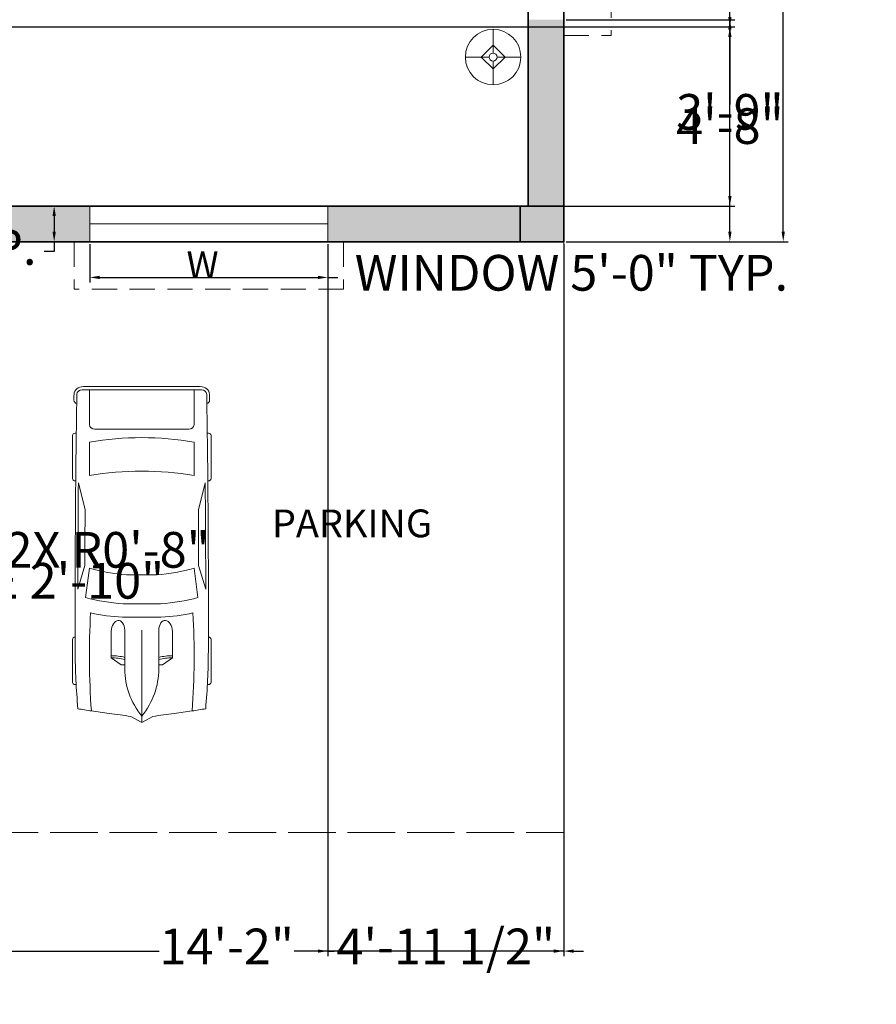
# Model space of a CAD drawing. Units: inches. Extents: x 9689 to 10369, y 10965 to 11626.
# Tile 9 of 11: x 10107 to 10323, y 10965 to 11214. Entities that reach past the tile are written whole.
import ezdxf

# ---------------------------------------------------------------- set-up
doc = ezdxf.new("R2010")
doc.units = ezdxf.units.IN
doc.linetypes.add('ACAD_ISO02W100', pattern=[15, 12, -3])
doc.linetypes.add('DASHED2', pattern=[9.525, 6.35, -3.175])
for name, color, linetype, lineweight in [('A-ANNO-DIMS', 2, 'Continuous', 18), ('A-ANNO-TEXT', 7, 'Continuous', 18), ('A-AREA-IDEN', 7, 'Continuous', 18), ('A-COLS', 7, 'Continuous', 35), ('A-FURN', 8, 'Continuous', 18), ('A-GLAZ', 4, 'Continuous', 18), ('A-GLAZ-OVHD', 4, 'DASHED2', 13), ('A-WALL', 7, 'Continuous', 35), ('A-WALL-PATT', 252, 'Continuous', 13), ('C-PARK', 7, 'ACAD_ISO02W100', 18), ('C-PARK-VEHI', 8, 'Continuous', 13)]:
    doc.layers.add(name, color=color, linetype=linetype, lineweight=lineweight)
doc.layers.add('A-COLS-PATT', color=18, linetype='Continuous', lineweight=13, true_color=0x000000)
doc.styles.get("Standard").update_dxf_attribs({"font": 'arial.ttf'})
doc.dimstyles.new('ISO-25', dxfattribs={"dimtxt": 9, "dimasz": 2.5, "dimexe": 1.25, "dimexo": 0.625, "dimgap": 2, "dimtad": 0, "dimtih": 1, "dimtoh": 1, "dimdec": 1, "dimlunit": 4, "dimtxsty": 'Standard', "dimcen": 2.5, "dimadec": 0, "dimazin": 0, "dimtfac": 0.5, "dimtdec": 1, "dimtmove": 0, "dimatfit": 3, "dimfxl": 1, "dimarcsym": 0})

# ---------------------------------------------------------------- blocks, each defined once
blk = doc.blocks.new('Lamp - Table')
for p, q in [((0, 7), (0, 1)), ((0, 3), (-3, 0)), ((3, 0), (0, 3)), ((-1, 0), (-7, 0)), ((-3, 0), (0, -3)), ((0, -3), (3, 0)), ((1, 0), (7, 0)), ((0, -1), (0, -7))]:
    blk.add_line(p, q)
for radius in [7, 1]:
    blk.add_circle((0, 0), radius)
blk = doc.blocks.new('*U18')
for p, q in [((1182, 988), (568, 988)), ((3472, 988), (4087, 988)), ((536, 950), (536, 936)), ((1214, 950), (1214, 950)), ((2235, 810), (1899, 912)), ((3412, 904), (3030, 807)), ((3440, 942), (3440, 950)), ((4119, 950), (4119, 934)), ((4736, -851), (4736, 851)), ((1779, 801), (2195, 746)), ((3516, 746), (3994, 746)), ((4736, 746), (4242, 746)), ((4785, -832), (4785, 832)), ((4179, 670), (4179, -670)), ((820, 295), (918, 436)), ((918, 436), (1294, 436)), ((816, 241), (816, 283)), ((83, 156), (3, 10)), ((756, 241), (1313, 241)), ((1496, -274), (1496, 274)), ((1690, -267), (1690, 267)), ((2102, 216), (2102, -216)), ((4736, -267), (4736, 267)), ((0, 0), (1313, 0)), ((3, -10), (83, -156)), ((756, -241), (1313, -241)), ((816, -241), (816, -283)), ((820, -295), (918, -436)), ((918, -436), (1294, -436)), ((2195, -746), (1779, -801)), ((2235, -810), (1899, -912)), ((3412, -904), (3030, -807)), ((3994, -746), (3516, -746)), ((4242, -746), (4736, -746)), ((536, -950), (536, -936)), ((1214, -950), (1214, -950)), ((3440, -942), (3440, -950)), ((4119, -950), (4119, -934)), ((1182, -988), (568, -988)), ((3472, -988), (4087, -988))]:
    blk.add_line(p, q)
for centre, major_axis, ratio, start_param, end_param in [((568, 950), (0, -37.6), 0.842304, 3.141593, 4.712389), ((1182, 950), (0, 37.6), 0.842304, -1.570796, 0), ((3472, 950), (0, -37.6), 0.842304, 3.141593, 4.712389), ((4087, 950), (0, 37.6), 0.842304, -1.570796, 0), ((6757, -699), (0, 7958), 0.842304, 1.367076, 1.39176), ((1046, -12468), (0, 13417), 0.842304, 0.00281, 0.075598), ((1638, -268113), (0, 269063), 0.842304, -0.013397, 0.002797), ((1638, -268113), (0, -269025), 0.842304, 3.133765, 3.140441), ((4588, 910), (0, 56.4), 0.842304, -0.013017, 1.249894), ((1638, -268131), (0, 269121), 0.842304, -0.013397, -0.013017), ((4673, 851), (0, -75.2), 0.842304, 1.570796, 3.128196), ((4673, 832), (0, -133), 0.842304, 1.570796, 3.128196), ((6583, -699), (0, -7755), 0.842304, 4.528606, 4.561838), ((952, -15087), (0, -15833), 0.842304, 3.096046, 3.200911), ((3414, 137), (0, -2280), 0.842304, 4.449482, 4.652344), ((3436, 137), (0, 2077), 0.842304, 1.245306, 1.50788), ((3800, 71), (0, -2021), 0.842304, 4.372215, 4.640744), ((2433, -93125), (0, -93935), 0.842304, 3.134049, 3.144098), ((434, 0), (0, 3734), 0.842304, 4.511394, 4.913384), ((912, 0), (0, 3734), 0.842304, 4.511394, 4.913384), ((4242, 670), (0, 75.2), 0.842304, 0, 1.570796), ((-5194, 1331), (0, -6374), 0.842304, 1.385369, 1.434372), ((331, 432), (0, 696), 0.842304, 4.435146, 4.718221), ((361, 432), (0, 696), 0.842304, 4.435146, 4.718221), ((1290, 339), (161, -9), 0.603834, -1.395552, 1.581315), ((832, 283), (0, 18.8), 0.842304, 0.879714, 1.570796), ((756, -1185), (0, 1427), 0.842304, 0, 0.590319), ((16, 0), (0, -18.8), 0.842304, 4.131459, 5.293319), ((756, 1185), (0, 1427), 0.842304, 2.551274, 3.141593), ((-5194, -1331), (0, 6374), 0.842304, -1.434372, -1.385369), ((331, -432), (0, -696), 0.842304, 1.564964, 1.848039), ((361, -432), (0, -696), 0.842304, 1.564964, 1.848039), ((3414, -137), (0, -2280), 0.842304, -1.510751, -1.307889), ((3436, -137), (0, -2077), 0.842304, -1.50788, -1.245306), ((3800, -71), (0, -2021), 0.842304, -1.499151, -1.230623), ((832, -283), (0, -18.8), 0.842304, 4.712389, 5.403472), ((6583, 699), (0, 7755), 0.842304, 1.721348, 1.754579), ((4242, -670), (0, -75.2), 0.842304, 4.712389, 6.283185), ((6757, 699), (0, 7958), 0.842304, 1.749832, 1.774517), ((952, 15087), (0, -15833), 0.842304, -0.059319, 0.045547), ((2433, 93125), (0, -93935), 0.842304, -0.002505, 0.007544), ((4673, -832), (0, -133), 0.842304, 0.013397, 1.570796), ((1046, 12468), (0, -13417), 0.842304, -0.075598, -0.00281), ((568, -950), (0, 37.6), 0.842304, 1.570796, 3.141593), ((1638, 268113), (0, 269063), 0.842304, 3.138796, 3.15499), ((1182, -950), (0, -37.6), 0.842304, 0, 1.570796), ((1638, 268113), (0, -269025), 0.842304, 0.001152, 0.007828), ((3472, -950), (0, -37.6), 0.842304, -1.570796, 0), ((4087, -950), (0, 37.6), 0.842304, 3.141593, 4.712389), ((4588, -910), (0, -56.4), 0.842304, -1.249894, 0.013017), ((1638, 268131), (0, 269121), 0.842304, 3.15461, 3.15499), ((4673, -851), (0, 75.2), 0.842304, 3.15499, 4.712389)]:
    blk.add_ellipse(centre, major_axis=major_axis, ratio=ratio, start_param=start_param, end_param=end_param)
at = {"extrusion": (0, 0, -1)}
blk.add_ellipse((1290, -339), major_axis=(161, 9), ratio=0.603834, start_param=-1.395552, end_param=1.581315, dxfattribs=at)
blk = doc.blocks.new('*D22')
at = {"layer": 'A-ANNO-DIMS', "color": 0, "lineweight": -2, "transparency": 16777216}
for p, q in [((10244.68, 11538.63), (10300.66, 11538.63)), ((10299.41, 11536.13), (10299.41, 11354.73)), ((10299.41, 11160.13), (10299.41, 11341.53)), ((10244.68, 11157.63), (10300.66, 11157.63))]:
    blk.add_line(p, q, dxfattribs=at)
at = {"layer": 'A-ANNO-DIMS', "color": 0, "transparency": 16777216}
for points in [[(10298.99, 11536.13), (10299.83, 11536.13), (10299.41, 11538.63)], [(10298.99, 11160.13), (10299.83, 11160.13), (10299.41, 11157.63)]]:
    blk.add_solid(points, dxfattribs=at)
at = {"layer": 'Defpoints', "color": 0, "transparency": 16777216}
for p in [(10244.06, 11538.63), (10244.06, 11157.63), (10299.41, 11157.63)]:
    blk.add_point(p, dxfattribs=at)
at = {"layer": 'A-ANNO-DIMS', "color": 0, "transparency": 16777216, "insert": (10299.41, 11348.13), "char_height": 9, "attachment_point": 5}
blk.add_mtext('31\'-9"', dxfattribs=at)
blk = doc.blocks.new('WINDOW-HOOD-68')
for p, q in [((12, 68), (0, 68)), ((0, 0), (0, 68)), ((12, 0), (0, 0))]:
    blk.add_line(p, q)
blk = doc.blocks.new('WINDOW-60')
for p, q in [((0, 60), (9, 60)), ((4.5, 60), (4.5, 0)), ((0, 0), (9, 0))]:
    blk.add_line(p, q)
blk = doc.blocks.new('*D40')
at = {"layer": 'A-ANNO-DIMS', "color": 0, "lineweight": -2, "transparency": 16777216}
for p, q in [((10124.56, 11157.01), (10124.56, 11147.38)), ((10184.56, 11157.01), (10184.56, 11147.38)), ((10127.06, 11148.63), (10182.06, 11148.63)), ((10184.56, 11148.63), (10187.06, 11148.63))]:
    blk.add_line(p, q, dxfattribs=at)
at = {"layer": 'A-ANNO-DIMS', "color": 0, "transparency": 16777216}
for points in [[(10127.06, 11149.05), (10127.06, 11148.21), (10124.56, 11148.63)], [(10182.06, 11149.05), (10182.06, 11148.21), (10184.56, 11148.63)]]:
    blk.add_solid(points, dxfattribs=at)
at = {"layer": 'Defpoints', "color": 0, "transparency": 16777216}
for p in [(10124.56, 11157.63), (10184.56, 11157.63), (10184.56, 11148.63)]:
    blk.add_point(p, dxfattribs=at)
at = {"layer": 'A-ANNO-DIMS', "color": 0, "transparency": 16777216, "insert": (10246, 11148.63), "char_height": 9, "attachment_point": 5}
blk.add_mtext('WINDOW 5\'-0" TYP.', dxfattribs=at)
blk = doc.blocks.new('*D41')
at = {"layer": 'A-ANNO-DIMS', "color": 0, "lineweight": -2, "transparency": 16777216}
for p, q in [((10123.93, 11166.63), (10114.31, 11166.63)), ((10115.56, 11164.13), (10115.56, 11160.13)), ((10123.93, 11157.63), (10114.31, 11157.63)), ((10115.56, 11157.63), (10115.56, 11155.13)), ((10115.56, 11155.13), (10113.06, 11155.13))]:
    blk.add_line(p, q, dxfattribs=at)
at = {"layer": 'A-ANNO-DIMS', "color": 0, "transparency": 16777216}
for points in [[(10115.14, 11164.13), (10115.97, 11164.13), (10115.56, 11166.63)], [(10115.14, 11160.13), (10115.97, 11160.13), (10115.56, 11157.63)]]:
    blk.add_solid(points, dxfattribs=at)
at = {"layer": 'Defpoints', "color": 0, "transparency": 16777216}
for p in [(10124.56, 11166.63), (10115.56, 11157.63), (10124.56, 11157.63)]:
    blk.add_point(p, dxfattribs=at)
at = {"layer": 'A-ANNO-DIMS', "color": 0, "transparency": 16777216, "insert": (10083.63, 11155.13), "char_height": 9, "attachment_point": 5}
blk.add_mtext('0\'-9" TYP.', dxfattribs=at)
blk = doc.blocks.new('*D62')
at = {"layer": 'A-ANNO-DIMS', "color": 0, "lineweight": -2, "transparency": 16777216}
for p, q in [((10087.02, 11087.95), (10081.3, 11087.95)), ((10082.55, 11085.45), (10082.55, 11077.6)), ((10082.55, 11056.45), (10082.55, 11064.29)), ((10087.02, 11053.95), (10081.3, 11053.95))]:
    blk.add_line(p, q, dxfattribs=at)
at = {"layer": 'A-ANNO-DIMS', "color": 0, "transparency": 16777216}
for points in [[(10082.13, 11085.45), (10082.96, 11085.45), (10082.55, 11087.95)], [(10082.13, 11056.45), (10082.96, 11056.45), (10082.55, 11053.95)]]:
    blk.add_solid(points, dxfattribs=at)
at = {"layer": 'Defpoints', "color": 0, "transparency": 16777216}
for p in [(10087.65, 11087.95), (10082.55, 11053.95), (10087.65, 11053.95)]:
    blk.add_point(p, dxfattribs=at)
at = {"layer": 'A-ANNO-DIMS', "color": 0, "transparency": 16777216, "insert": (10082.55, 11070.95), "char_height": 9, "attachment_point": 5}
blk.add_mtext('EXERCISE BIKE 2\'-10"', dxfattribs=at)
blk = doc.blocks.new('*D74')
at = {"layer": 'A-ANNO-DIMS', "color": 0, "lineweight": -2, "transparency": 16777216}
for p, q in [((10285.96, 11221.79), (10285.96, 11224.29)), ((10285.96, 11224.29), (10288.46, 11224.29)), ((10068.68, 11221.79), (10287.21, 11221.79)), ((10285.96, 11214.29), (10285.96, 11219.29)), ((10068.68, 11211.79), (10287.21, 11211.79))]:
    blk.add_line(p, q, dxfattribs=at)
at = {"layer": 'A-ANNO-DIMS', "color": 0, "transparency": 16777216}
for points in [[(10285.54, 11219.29), (10286.37, 11219.29), (10285.96, 11221.79)], [(10285.54, 11214.29), (10286.37, 11214.29), (10285.96, 11211.79)]]:
    blk.add_solid(points, dxfattribs=at)
at = {"layer": 'Defpoints', "color": 0, "transparency": 16777216}
for p in [(10068.06, 11221.79), (10285.96, 11221.79), (10068.06, 11211.79)]:
    blk.add_point(p, dxfattribs=at)
at = {"layer": 'A-ANNO-DIMS', "color": 0, "transparency": 16777216, "insert": (10305.92, 11224.29), "char_height": 9, "attachment_point": 5}
blk.add_mtext('0\'-10"', dxfattribs=at)
blk = doc.blocks.new('*D75')
at = {"layer": 'A-ANNO-DIMS', "color": 0, "lineweight": -2, "transparency": 16777216}
for p, q in [((10068.68, 11211.79), (10287.21, 11211.79)), ((10285.96, 11209.29), (10285.96, 11195.81)), ((10285.96, 11169.13), (10285.96, 11182.61)), ((10068.68, 11166.63), (10287.21, 11166.63))]:
    blk.add_line(p, q, dxfattribs=at)
at = {"layer": 'A-ANNO-DIMS', "color": 0, "transparency": 16777216}
for points in [[(10285.54, 11209.29), (10286.37, 11209.29), (10285.96, 11211.79)], [(10285.54, 11169.13), (10286.37, 11169.13), (10285.96, 11166.63)]]:
    blk.add_solid(points, dxfattribs=at)
at = {"layer": 'Defpoints', "color": 0, "transparency": 16777216}
for p in [(10068.06, 11211.79), (10285.96, 11211.79), (10068.06, 11166.63)]:
    blk.add_point(p, dxfattribs=at)
at = {"layer": 'A-ANNO-DIMS', "color": 0, "transparency": 16777216, "insert": (10285.96, 11189.21), "char_height": 9, "attachment_point": 5}
blk.add_mtext('3\'-9"', dxfattribs=at)
blk = doc.blocks.new('*D96')
at = {"layer": 'A-ANNO-DIMS', "color": 0, "lineweight": -2, "transparency": 16777216}
for p, q in [((10074.06, 11075.01), (10074.06, 10977.48)), ((10244.06, 11008.01), (10244.06, 10977.48)), ((10076.56, 10978.73), (10142.02, 10978.73)), ((10241.56, 10978.73), (10176.09, 10978.73))]:
    blk.add_line(p, q, dxfattribs=at)
at = {"layer": 'A-ANNO-DIMS', "color": 0, "transparency": 16777216}
for points in [[(10076.56, 10979.15), (10076.56, 10978.31), (10074.06, 10978.73)], [(10241.56, 10979.15), (10241.56, 10978.31), (10244.06, 10978.73)]]:
    blk.add_solid(points, dxfattribs=at)
at = {"layer": 'Defpoints', "color": 0, "transparency": 16777216}
for p in [(10074.06, 11075.63), (10244.06, 11008.63), (10244.06, 10978.73)]:
    blk.add_point(p, dxfattribs=at)
at = {"layer": 'A-ANNO-DIMS', "color": 0, "transparency": 16777216, "insert": (10159.06, 10978.73), "char_height": 9, "attachment_point": 5}
blk.add_mtext('14\'-2"', dxfattribs=at)
blk = doc.blocks.new('*D102')
at = {"layer": 'A-ANNO-DIMS', "color": 0, "lineweight": -2, "transparency": 16777216}
for p, q in [((10184.56, 11157.01), (10184.56, 10977.48)), ((10244.06, 11157.01), (10244.06, 10977.48)), ((10182.06, 10978.73), (10179.56, 10978.73)), ((10184.56, 10978.73), (10186.18, 10978.73)), ((10244.06, 10978.73), (10242.43, 10978.73)), ((10246.56, 10978.73), (10249.06, 10978.73))]:
    blk.add_line(p, q, dxfattribs=at)
at = {"layer": 'A-ANNO-DIMS', "color": 0, "transparency": 16777216}
for points in [[(10182.06, 10979.15), (10182.06, 10978.31), (10184.56, 10978.73)], [(10246.56, 10979.15), (10246.56, 10978.31), (10244.06, 10978.73)]]:
    blk.add_solid(points, dxfattribs=at)
at = {"layer": 'Defpoints', "color": 0, "transparency": 16777216}
for p in [(10184.56, 11157.63), (10244.06, 11157.63), (10244.06, 10978.73)]:
    blk.add_point(p, dxfattribs=at)
at = {"layer": 'A-ANNO-DIMS', "color": 0, "transparency": 16777216, "insert": (10214.31, 10978.73), "char_height": 9, "attachment_point": 5}
blk.add_mtext('4\'-11 1/2"', dxfattribs=at)
blk = doc.blocks.new('*D103')
at = {"layer": 'A-ANNO-DIMS', "color": 0, "lineweight": -2, "transparency": 16777216}
for p, q in [((10244.68, 11213.63), (10287.21, 11213.63)), ((10285.96, 11211.13), (10285.96, 11192.23)), ((10285.96, 11160.13), (10285.96, 11179.03)), ((10244.68, 11157.63), (10287.21, 11157.63))]:
    blk.add_line(p, q, dxfattribs=at)
at = {"layer": 'A-ANNO-DIMS', "color": 0, "transparency": 16777216}
for points in [[(10285.54, 11211.13), (10286.37, 11211.13), (10285.96, 11213.63)], [(10285.54, 11160.13), (10286.37, 11160.13), (10285.96, 11157.63)]]:
    blk.add_solid(points, dxfattribs=at)
at = {"layer": 'Defpoints', "color": 0, "transparency": 16777216}
for p in [(10244.06, 11213.63), (10285.96, 11213.63), (10244.06, 11157.63)]:
    blk.add_point(p, dxfattribs=at)
at = {"layer": 'A-ANNO-DIMS', "color": 0, "transparency": 16777216, "insert": (10285.96, 11185.63), "char_height": 9, "attachment_point": 5}
blk.add_mtext('4\'-8"', dxfattribs=at)
blk = doc.blocks.new('*D107')
at = {"layer": 'A-ANNO-DIMS', "color": 0, "lineweight": -2, "transparency": 16777216}
for p, q in [((10235.68, 11320.63), (10287.21, 11320.63)), ((10285.96, 11318.13), (10285.96, 11250.23)), ((10285.96, 11169.13), (10285.96, 11237.03)), ((10235.68, 11166.63), (10287.21, 11166.63))]:
    blk.add_line(p, q, dxfattribs=at)
at = {"layer": 'A-ANNO-DIMS', "color": 0, "transparency": 16777216}
for points in [[(10285.54, 11318.13), (10286.37, 11318.13), (10285.96, 11320.63)], [(10285.54, 11169.13), (10286.37, 11169.13), (10285.96, 11166.63)]]:
    blk.add_solid(points, dxfattribs=at)
at = {"layer": 'Defpoints', "color": 0, "transparency": 16777216}
for p in [(10235.06, 11320.63), (10285.96, 11320.63), (10235.06, 11166.63)]:
    blk.add_point(p, dxfattribs=at)
at = {"layer": 'A-ANNO-DIMS', "color": 0, "transparency": 16777216, "insert": (10285.96, 11243.63), "char_height": 9, "attachment_point": 5}
blk.add_mtext('12\'-10"', dxfattribs=at)
blk = doc.blocks.new('*D130')
at = {"layer": 'A-ANNO-DIMS', "color": 0, "lineweight": -2, "transparency": 16777216}
for p, q in [((10098.52, 11078.76), (10096.29, 11077.64)), ((10101.02, 11078.76), (10098.52, 11078.76)), ((10086.73, 11072.86), (10094.05, 11076.52))]:
    blk.add_line(p, q, dxfattribs=at)
at = {"layer": 'A-ANNO-DIMS', "color": 0, "transparency": 16777216}
blk.add_solid([(10096.1, 11078.02), (10096.47, 11077.27), (10094.05, 11076.52)], dxfattribs=at)
at = {"layer": 'Defpoints', "color": 0, "transparency": 16777216}
for p in [(10094.05, 11076.52), (10086.73, 11072.86)]:
    blk.add_point(p, dxfattribs=at)
at = {"layer": 'A-ANNO-DIMS', "color": 0, "transparency": 16777216, "insert": (10129.04, 11078.76), "char_height": 9, "attachment_point": 5}
blk.add_mtext('2X R0\'-8"', dxfattribs=at)

msp = doc.modelspace()

# ---------------------------------------------------------------- hatches: boundary and pattern name
at = {"layer": 'A-COLS-PATT'}
h = msp.add_hatch(color=256, dxfattribs=at)
h.dxf.hatch_style = 1
h.paths.add_polyline_path([(10244.06, 11166.63), (10235.06, 11166.63), (10233.06, 11166.63), (10233.06, 11157.63), (10244.06, 11157.63)])
at = {"layer": 'A-WALL-PATT'}
h = msp.add_hatch(dxfattribs=at)
h.set_pattern_fill('ANSI36', color=256)
h.paths.add_polyline_path([(10233.06, 11326.63), (10173.19, 11326.63, -0.055385), (10173.19, 11320.63), (10233.06, 11320.63)])
h.paths.add_polyline_path([(10244.06, 11213.63), (10235.06, 11213.63), (10235.06, 11166.63), (10244.06, 11166.63)])
h.paths.add_polyline_path([(10233.06, 11166.63), (10184.56, 11166.63), (10184.56, 11157.63), (10233.06, 11157.63)])
h.paths.add_polyline_path([(10124.56, 11166.63), (10074.06, 11166.63), (10074.06, 11157.63), (10124.56, 11157.63)])
h.paths.add_polyline_path([(10074.06, 11318.63), (10068.06, 11318.63), (10068.06, 11168.63), (10074.06, 11168.63)])
h.paths.add_polyline_path([(10068.06, 11166.63), (10011.06, 11166.63), (10011.06, 11157.63), (10068.06, 11157.63)])
h.paths.add_polyline_path([(10011.06, 11318.63), (10005.06, 11318.63), (10005.06, 11168.63), (10011.06, 11168.63)])
h.paths.add_polyline_path([(10005.06, 11166.63), (9985.06, 11166.63), (9985.06, 11157.63), (10005.06, 11157.63)])
h.paths.add_polyline_path([(9937.06, 11166.63), (9898.06, 11166.63), (9898.06, 11157.63), (9937.06, 11157.63, -0.042779)])
h.paths.add_polyline_path([(9850.06, 11166.63), (9813.06, 11166.63), (9813.06, 11157.63), (9850.06, 11157.63)])
h.paths.add_polyline_path([(9811.06, 11213.63), (9802.06, 11213.63), (9802.06, 11166.63), (9811.06, 11166.63)])
h.paths.add_polyline_path([(9811.06, 11320.63), (9802.06, 11320.63), (9802.06, 11273.63), (9811.06, 11273.63)])
h.paths.add_polyline_path([(9811.06, 11439.11), (9802.06, 11439.11), (9802.06, 11326.63), (9811.06, 11326.63)])
h.paths.add_polyline_path([(9957.06, 11326.63), (9813.06, 11326.63), (9813.06, 11320.63), (9957.06, 11320.63)])
h.paths.add_polyline_path([(9811.06, 11527.63), (9802.06, 11527.63), (9802.06, 11499.11), (9811.06, 11499.11)])

# ---------------------------------------------------------------- linework, layer by layer
at = {"layer": 'A-COLS'}
for p, q in [((10233.06, 11166.63), (10233.06, 11157.63)), ((10235.06, 11166.63), (10244.06, 11166.63))]:
    msp.add_line(p, q, dxfattribs=at)
at = {"layer": 'A-WALL'}
for p, q in [((10244.06, 11538.63), (10244.06, 11157.63)), ((10235.06, 11320.63), (10235.06, 11166.63)), ((10235.06, 11166.63), (10074.06, 11166.63)), ((10244.06, 11157.63), (9985.06, 11157.63))]:
    msp.add_line(p, q, dxfattribs=at)
at = {"layer": 'C-PARK'}
for p in [(10244.06, 11157.63), (9904.55, 11008.63)]:
    msp.add_line(p, (10244.06, 11008.63), dxfattribs=at)

# ---------------------------------------------------------------- block references
at = {"layer": 'A-FURN'}
msp.add_blockref('Lamp - Table', (10226.25, 11204.2), dxfattribs=at)
at = {"layer": 'A-GLAZ', "rotation": 269.9999999999898}
msp.add_blockref('WINDOW-60', (10124.56, 11166.63), dxfattribs=at)
at = {"layer": 'A-GLAZ-OVHD'}
for p, rotation in [((10256.06, 11277.63), 180), ((10188.56, 11145.63), 89.99999999998991)]:
    msp.add_blockref('WINDOW-HOOD-68', p, dxfattribs=dict(at, rotation=rotation))
at = {"layer": 'C-PARK-VEHI', "xscale": 0.0176923662941297, "yscale": 0.0176923662941297, "zscale": 0.0176923662941297, "rotation": 90}
msp.add_blockref('*U18', (10137.65, 11036.45), dxfattribs=at)

# ---------------------------------------------------------------- texts
at = {"layer": 'A-ANNO-TEXT', "insert": (10148.95, 11155.17), "char_height": 6.729, "attachment_point": 1}
msp.add_mtext_dynamic_manual_height_columns('{\\fArial|b1|i0|c0|p34;W}', width=31.3623, gutter_width=33.65, heights=[0], dxfattribs=at)
at = {"layer": 'A-AREA-IDEN', "insert": (10170.47, 11090.1), "char_height": 7, "attachment_point": 1}
msp.add_mtext_dynamic_manual_height_columns('{\\fArial|b1|i0|c0|p34;PARKING}', width=67.3152, gutter_width=12.5, heights=[0], dxfattribs=at)

# ---------------------------------------------------------------- dimensions: what is measured, and where the dimension line sits
at = {"layer": 'A-ANNO-DIMS'}
for base, p1, p2, override, picture, middle in [((10299.41, 11157.63), (10244.06, 11538.63), (10244.06, 11157.63), {"dimclrd": 0, "dimclre": 0, "dimclrt": 0}, '*D22', (10299.41, 11348.13)), ((10285.96, 11320.63), (10235.06, 11166.63), (10235.06, 11320.63), {"dimdec": 1, "dimlfac": 1, "dimrnd": 0, "dimzin": 1, "dimdsep": 46, "dimlunit": 4, "dimfrac": 2}, '*D107', (10285.96, 11243.63)), ((10285.96, 11221.79), (10068.06, 11211.79), (10068.06, 11221.79), {"dimdec": 1, "dimlfac": 1, "dimrnd": 0, "dimzin": 1, "dimdsep": 46, "dimlunit": 4, "dimfrac": 2}, '*D74', (10305.92, 11224.29)), ((10285.96, 11211.79), (10068.06, 11166.63), (10068.06, 11211.79), {"dimdec": 1, "dimlfac": 1, "dimrnd": 0, "dimzin": 1, "dimdsep": 46, "dimlunit": 4, "dimfrac": 2}, '*D75', (10285.96, 11189.21)), ((10285.96, 11213.63), (10244.06, 11157.63), (10244.06, 11213.63), {"dimdec": 1, "dimlfac": 1, "dimrnd": 0, "dimzin": 1, "dimdsep": 46, "dimlunit": 4, "dimfrac": 2}, '*D103', (10285.96, 11185.63))]:
    dim = msp.add_linear_dim(base=base, p1=p1, p2=p2, angle=90, dimstyle='ISO-25', override=override, dxfattribs=at)
    dim.commit()
    dim.dimension.update_dxf_attribs({"geometry": picture, "text_midpoint": middle})
dim = msp.add_linear_dim(base=(10184.56, 11148.63), p1=(10124.56, 11157.63), p2=(10184.56, 11157.63), text='WINDOW <> TYP.', dimstyle='ISO-25', override={"dimdec": 1, "dimlfac": 1, "dimrnd": 0, "dimzin": 1, "dimdsep": 46, "dimlunit": 4, "dimfrac": 2}, dxfattribs=at)
dim.commit()
dim.dimension.update_dxf_attribs({"geometry": '*D40', "text_midpoint": (10246, 11148.63)})
for base, p1, p2, text, picture, middle in [((10115.56, 11157.63), (10124.56, 11166.63), (10124.56, 11157.63), '<> TYP.', '*D41', (10083.63, 11155.13)), ((10082.55, 11053.95), (10087.65, 11087.95), (10087.65, 11053.95), 'EXERCISE BIKE <>', '*D62', (10082.55, 11070.95))]:
    dim = msp.add_linear_dim(base=base, p1=p1, p2=p2, angle=270, text=text, dimstyle='ISO-25', override={"dimdec": 1, "dimlfac": 1, "dimrnd": 0, "dimzin": 1, "dimdsep": 46, "dimlunit": 4, "dimfrac": 2}, dxfattribs=at)
    dim.commit()
    dim.dimension.update_dxf_attribs({"geometry": picture, "text_midpoint": middle})
for p1, p2, picture, middle in [((10184.56, 11157.63), (10244.06, 11157.63), '*D102', (10214.31, 10978.73)), ((10074.06, 11075.63), (10244.06, 11008.63), '*D96', (10159.06, 10978.73))]:
    dim = msp.add_linear_dim(base=(10244.06, 10978.73), p1=p1, p2=p2, dimstyle='ISO-25', override={"dimdec": 1, "dimlfac": 1, "dimrnd": 0, "dimzin": 1, "dimdsep": 46, "dimlunit": 4, "dimfrac": 2}, dxfattribs=at)
    dim.commit()
    dim.dimension.update_dxf_attribs({"geometry": picture, "text_midpoint": middle})
dim = msp.add_radius_dim(center=(10086.73, 11072.86), mpoint=(10094.05, 11076.52), text='2X <>', dimstyle='ISO-25', override={"dimdec": 1, "dimlfac": 1, "dimrnd": 0, "dimzin": 1, "dimdsep": 46, "dimlunit": 4, "dimfrac": 2}, dxfattribs=at)
dim.commit()
dim.dimension.update_dxf_attribs({"geometry": '*D130', "text_midpoint": (10129.04, 11078.76)})

doc.saveas('drawing.dxf')
